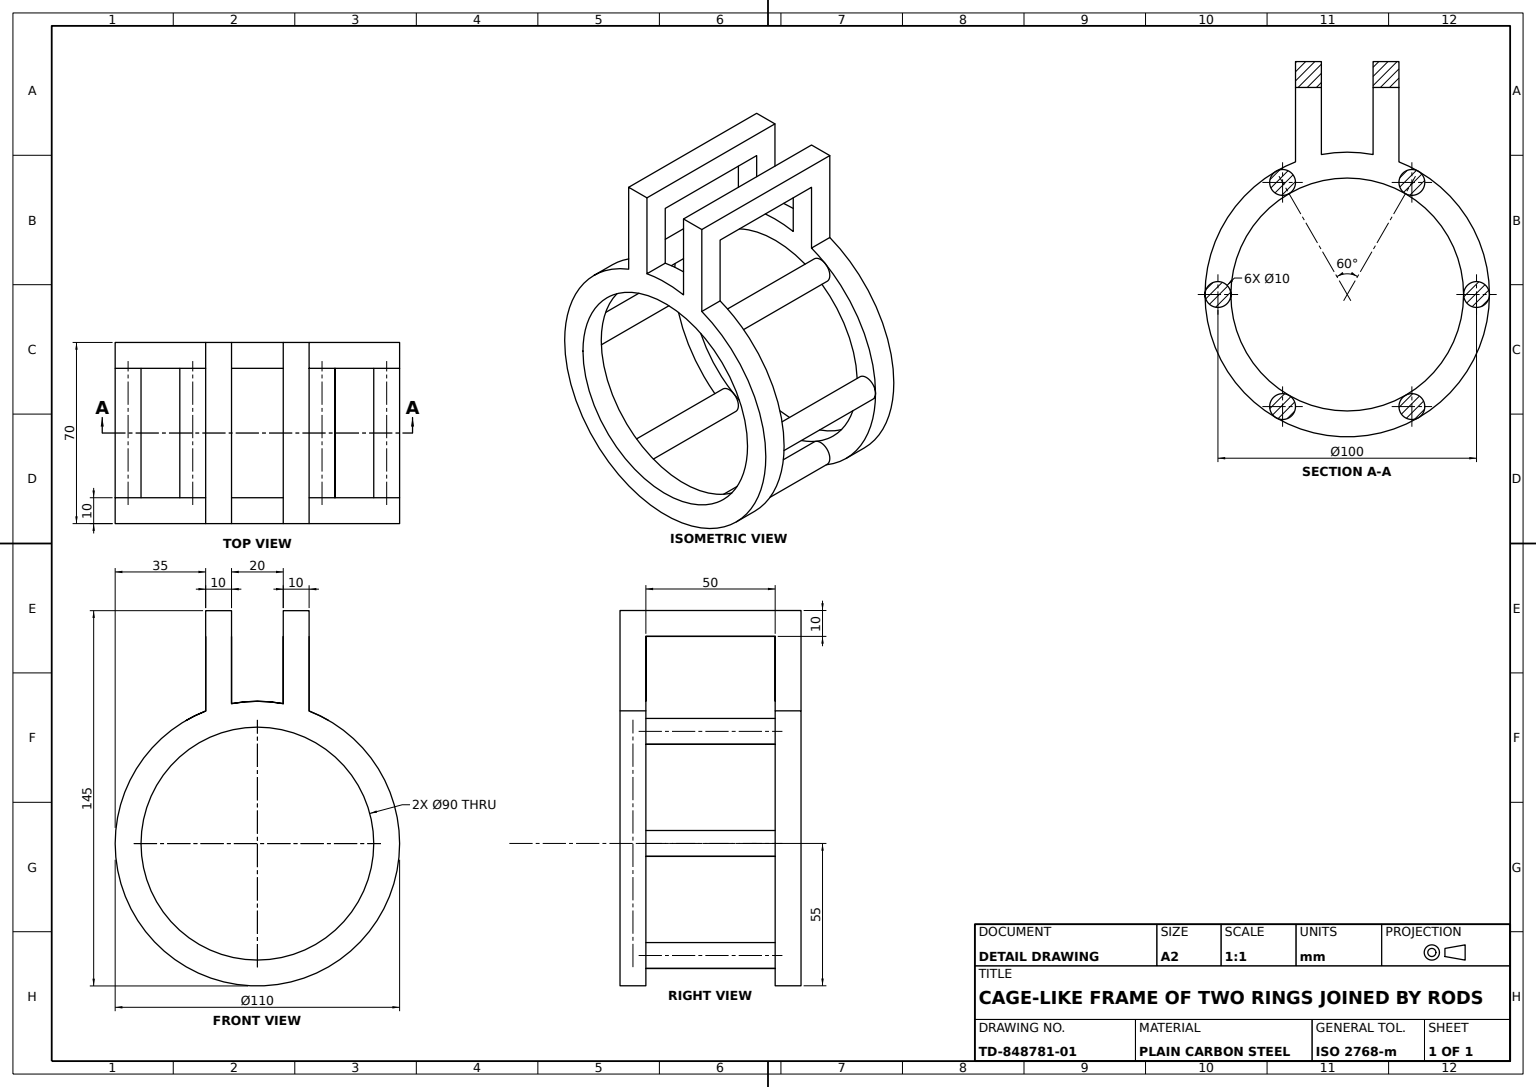
from build123d import *

# Parameters (mm, degrees)
FRONT_RING_PROFILE_110_R  = 55
FRONT_RING_DISC_DEPTH     = 10
REAR_RING_PROFILE_R       = 55
REAR_RING_DISC_DEPTH      = 10
RING_BORE_90_PROFILE_R    = 45
RING_BORE_90_DEPTH        = 105.642247682
FRONT_CLAMP_BRACKET_DEPTH = 10
REAR_CLAMP_BRACKET_DEPTH  = 10
CAGE_RODS_6X_10_PROFILE_R = 5
CAGE_RODS_6X_10_DEPTH     = 50


with BuildPart() as part:
    # Front Ring Profile Ø110 → Front Ring Disc (new body)
    with BuildSketch(Plane.XY):
        Circle(FRONT_RING_PROFILE_110_R)
    extrude(amount=-FRONT_RING_DISC_DEPTH)


with BuildPart() as body_2:
    # Rear Ring Profile → Rear Ring Disc (new body)
    with BuildSketch(Plane.XY.offset(-70)):
        Circle(REAR_RING_PROFILE_R)
    extrude(amount=REAR_RING_DISC_DEPTH)


with BuildPart() as ring_bore_90_tool:
    # Ring Bore Ø90 Profile → Ring Bore Ø90 (new, through all)
    with BuildSketch(Plane.XY):
        Circle(RING_BORE_90_PROFILE_R)
    extrude(amount=-RING_BORE_90_DEPTH)


with BuildPart() as part_1:
    add(part.part)

    # Ring Bore Ø90: cut by ring_bore_90_tool
    add(ring_bore_90_tool.part, mode=Mode.SUBTRACT)



with BuildPart() as body_2_1:
    add(body_2.part)

    # Ring Bore Ø90: cut by ring_bore_90_tool
    add(ring_bore_90_tool.part, mode=Mode.SUBTRACT)


with BuildPart() as part_2:
    add(part_1.part)

    add(body_2_1.part)  # Front Clamp Bracket merges body 2
    # Front Clamp Bracket Profile → Front Clamp Bracket (add)
    with BuildSketch(Plane(origin=(20, 0, 0), x_dir=(0, 0, -1), z_dir=(1, 0, 0))):
        Polygon((0, 45), (0, 90), (70, 90), (70, 45), (60, 45), (60, 80), (10, 80), (10, 45), align=None)
    extrude(amount=-FRONT_CLAMP_BRACKET_DEPTH)

    # Rear Clamp Bracket Profile → Rear Clamp Bracket (add)
    with BuildSketch(Plane(origin=(-20, 0, 0), x_dir=(0, 0, -1), z_dir=(1, 0, 0))):
        Polygon((10, 80), (60, 80), (60, 51.23475383), (70, 51.23475383), (70, 90), (0, 90), (0, 51.23475383), (10, 51.23475383), align=None)
    extrude(amount=REAR_CLAMP_BRACKET_DEPTH)

    # Cage Rods 6xØ10 Profile → Cage Rods 6xØ10 (add)
    with BuildSketch(Plane(origin=(0, 0, -10), x_dir=(-1, 0, 0), z_dir=(0, 0, -1))):
        with Locations(Location((50, 0, 0), (0, 0, 180))):
            Circle(CAGE_RODS_6X_10_PROFILE_R)
        with Locations(Location((25, -43.301270189, 0), (0, 0, 120))):
            Circle(CAGE_RODS_6X_10_PROFILE_R)
        with Locations(Location((-25, -43.301270189, 0), (0, 0, 240))):
            Circle(CAGE_RODS_6X_10_PROFILE_R)
        with Locations(Location((-50, 0, 0), (0, 0, 180))):
            Circle(CAGE_RODS_6X_10_PROFILE_R)
        with Locations(Location((-25, 43.301270189, 0), (0, 0, 120))):
            Circle(CAGE_RODS_6X_10_PROFILE_R)
        with Locations(Location((25, 43.301270189, 0), (0, 0, 240))):
            Circle(CAGE_RODS_6X_10_PROFILE_R)
    extrude(amount=CAGE_RODS_6X_10_DEPTH)


solid = part_2.part
